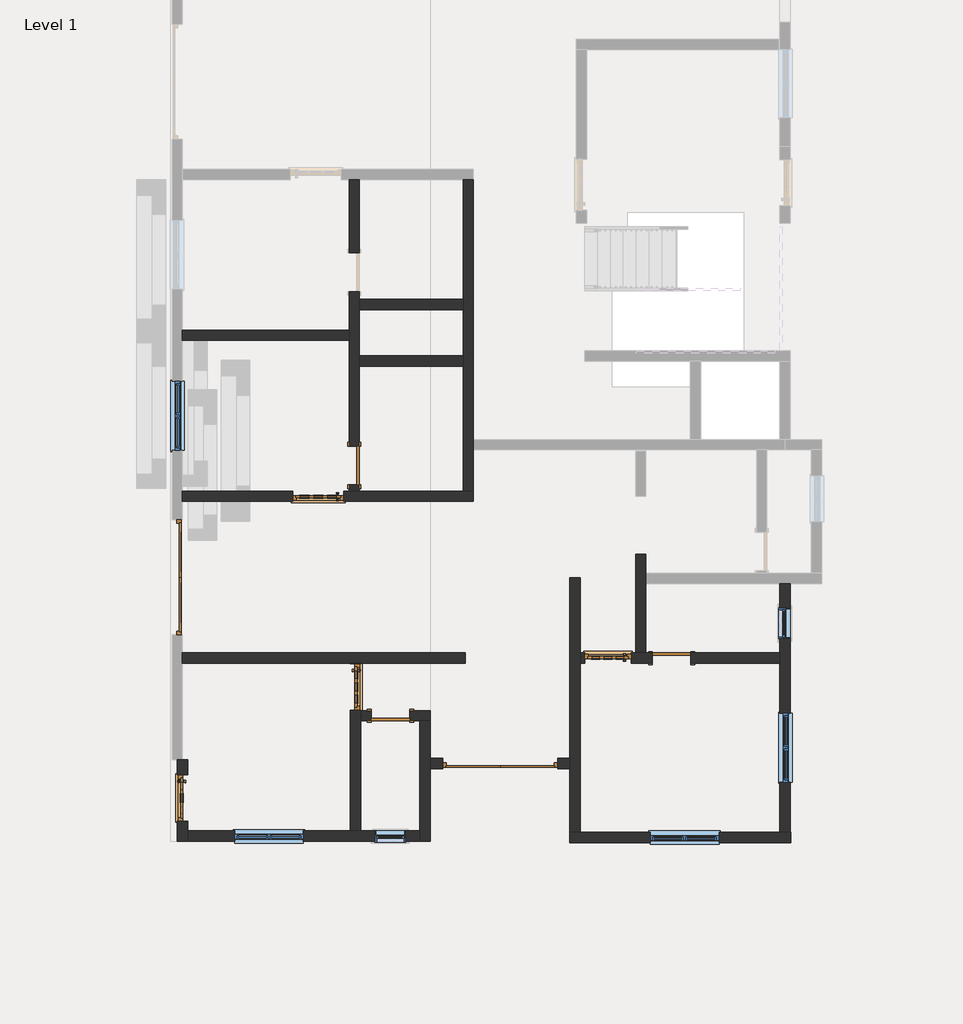
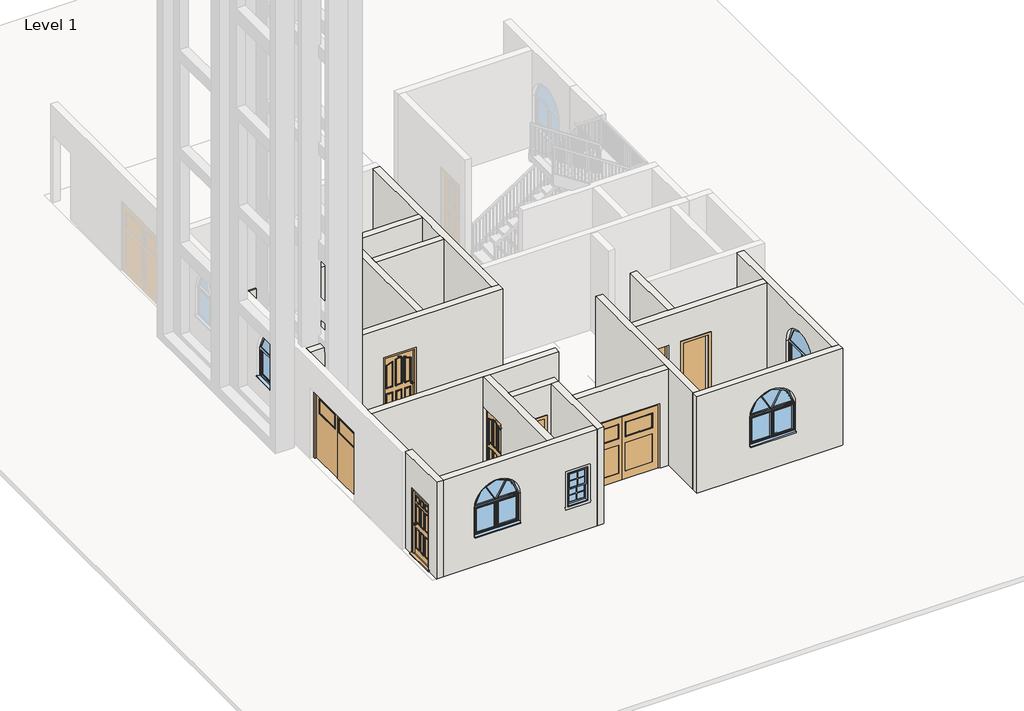
# One storey, part 1 of 4: 18 walls, 9 doors, 6 windows.
"""IFC4 building model written with IfcOpenShell, lengths in millimetres."""

from ifc_helpers import new_model, si_unit, frame, origin, origin_with_axes, place, context, project, spatial, polyline, circle_curve, outline, extrude, faceted_brep, transform, mapped, element, save
from ifc_brep_helpers import plane_surface, revolved_surface, advanced_brep
from components import doors_extsgl_5_910x2110mm_99758a98, doors_extsgl_6_1010x2110mm_b93c615f, doors_extsgl_6_1010x2110mm_efbaf1af, doors_extsgl_6_910x2110mm_72be2df1, doors_extsgl_6_910x2110mm_b26fcae4, doors_extsgl_6_910x2110mm_5dc58899, doors_extsgl_6_910x2110mm_16d7c084, doors_garage_timber_side_hung_glazing_2270x2050mm_ae99176d, doors_garage_timber_side_hung_glazing_2270x2200mm_badb7014, door_fadea3f2, door_53b1b562, window_679d2811, windows_arched_1360x910mm_c5754810

model = new_model("IFC4")

# Units and contexts
model_context = context("Model", 3, world=origin())
ifc_project = project(units=[si_unit("LENGTHUNIT", "METRE", prefix="MILLI")], contexts=[model_context])

# Site, building, storey
site = spatial("IfcSite", under=ifc_project)
building = spatial("IfcBuilding", under=site)
storey = spatial("IfcBuildingStorey", under=building, Name="Level 1", Elevation=0.0)

# Doors
placement = place(None, origin())
doors_extsgl_5_910x2110mm_shape = doors_extsgl_5_910x2110mm_99758a98(model_context)
element("IfcDoor", 1, ObjectType="Doors_ExtSgl_5 : 910x2110mm", at=placement, inside=storey, context=model_context, shape_type="MappedRepresentation", body=[
    mapped(doors_extsgl_5_910x2110mm_shape, transform((-6127.6013636, -9759.5108149, 0.0), x_axis=(0.0, -1.0, 0.0), y_axis=(1.0, 0.0, 0.0), z_axis=(0.0, 0.0, 1.0))),
])
doors_extsgl_6_1010x2110mm_shape = doors_extsgl_6_1010x2110mm_b93c615f(model_context)
doors_extsgl_6_1010x2110mm_2_shape = doors_extsgl_6_1010x2110mm_efbaf1af(model_context)
element("IfcDoor", 2, ObjectType="Doors_ExtSgl_6 : 1010x2110mm", at=placement, inside=storey, context=model_context, shape_type="MappedRepresentation", body=[
    mapped(doors_extsgl_6_1010x2110mm_shape, transform((-3445.8775704, -3805.7037749, 0.0), x_axis=(-1.0, 0.0, 0.0), y_axis=(0.0, -1.0, 0.0), z_axis=(0.0, 0.0, 1.0))),
    mapped(doors_extsgl_6_1010x2110mm_2_shape, transform((-3445.8775704, -3805.7037749, 0.0), x_axis=(-1.0, 0.0, 0.0), y_axis=(0.0, -1.0, 0.0), z_axis=(0.0, 0.0, 1.0))),
])
doors_extsgl_6_910x2110mm_shape = doors_extsgl_6_910x2110mm_72be2df1(model_context)
doors_extsgl_6_910x2110mm_2_shape = doors_extsgl_6_910x2110mm_b26fcae4(model_context)
element("IfcDoor", 3, ObjectType="Doors_ExtSgl_6 : 910x2110mm", at=placement, inside=storey, context=model_context, shape_type="MappedRepresentation", body=[
    mapped(doors_extsgl_6_910x2110mm_shape, transform((2269.1224296, -6998.5466225, 0.0), x_axis=(-1.0, 0.0, 0.0), y_axis=(0.0, -1.0, 0.0), z_axis=(0.0, 0.0, 1.0))),
    mapped(doors_extsgl_6_910x2110mm_2_shape, transform((2269.1224296, -6998.5466225, 0.0), x_axis=(-1.0, 0.0, 0.0), y_axis=(0.0, -1.0, 0.0), z_axis=(0.0, 0.0, 1.0))),
])
doors_extsgl_6_910x2110mm_3_shape = doors_extsgl_6_910x2110mm_5dc58899(model_context)
doors_extsgl_6_910x2110mm_4_shape = doors_extsgl_6_910x2110mm_16d7c084(model_context)
element("IfcDoor", 4, ObjectType="Doors_ExtSgl_6 : 910x2110mm", at=placement, inside=storey, context=model_context, shape_type="MappedRepresentation", body=[
    mapped(doors_extsgl_6_910x2110mm_3_shape, transform((-2709.3109037, -7568.3747197, 0.0), x_axis=(0.0, -1.0, 0.0), y_axis=(1.0, 0.0, 0.0), z_axis=(0.0, 0.0, 1.0))),
    mapped(doors_extsgl_6_910x2110mm_4_shape, transform((-2709.3109037, -7568.3747197, 0.0), x_axis=(0.0, -1.0, 0.0), y_axis=(1.0, 0.0, 0.0), z_axis=(0.0, 0.0, 1.0))),
])
doors_garage_timber_side_hung_glazing_2270x2050mm_shape = doors_garage_timber_side_hung_glazing_2270x2050mm_ae99176d(model_context)
element("IfcDoor", 5, ObjectType="Doors_Garage_Timber_Side_Hung_Glazing : 2270x2050mm", at=placement, inside=storey, context=model_context, shape_type="MappedRepresentation", body=[
    mapped(doors_garage_timber_side_hung_glazing_2270x2050mm_shape, transform((141.8390963, -9078.0694836, 0.0), x_axis=(-1.0, 0.0, 0.0), y_axis=(0.0, -1.0, 0.0), z_axis=(0.0, 0.0, 1.0))),
])
doors_garage_timber_side_hung_glazing_2270x2200mm_shape = doors_garage_timber_side_hung_glazing_2270x2200mm_badb7014(model_context)
element("IfcDoor", 6, ObjectType="Doors_Garage_Timber_Side_Hung_Glazing : 2270x2200mm", at=placement, inside=storey, context=model_context, shape_type="MappedRepresentation", body=[
    mapped(doors_garage_timber_side_hung_glazing_2270x2200mm_shape, transform((-6229.2013636, -5402.1251987, 0.0), x_axis=(0.0, 1.0, 0.0), y_axis=(-1.0, 0.0, 0.0), z_axis=(0.0, 0.0, 1.0))),
])
door_shape = door_fadea3f2(model_context)
element("IfcDoor", 7, ObjectType="Single-Flush : 30\" x 80\"", at=placement, inside=storey, context=model_context, shape_type="MappedRepresentation", body=[
    mapped(door_shape, transform((-2023.5109037, -8138.2694836, 0.0), x_axis=(-1.0, 0.0, 0.0), y_axis=(0.0, -1.0, 0.0), z_axis=(0.0, 0.0, 1.0))),
])
door_2_shape = door_53b1b562(model_context)
element("IfcDoor", 8, ObjectType="Single-Flush : 30\" x 80\"", at=placement, inside=storey, context=model_context, shape_type="MappedRepresentation", body=[
    mapped(door_2_shape, transform((-2734.7109037, -3196.1037749, 0.0), x_axis=(0.0, 1.0, 0.0), y_axis=(-1.0, 0.0, 0.0), z_axis=(0.0, 0.0, 1.0))),
])
element("IfcDoor", 9, ObjectType="Single-Flush : 30\" x 80\"", at=placement, inside=storey, context=model_context, shape_type="MappedRepresentation", body=[
    mapped(door_2_shape, transform((3526.3890963, -6998.5466225, 0.0), x_axis=(-1.0, 0.0, 0.0), y_axis=(0.0, -1.0, 0.0), z_axis=(0.0, 0.0, 1.0))),
])

# Walls
element("IfcWall", 10, ObjectType="Generic - 9\" w", at=placement, inside=storey, context=model_context, shape_type="AdvancedBrep", body=[
    advanced_brep(
    [(1519.7890963, -10638.3037749, 0.0), (5875.8890963, -10638.3037749, 0.0), (5875.8890963, -10638.3037749, 3048.0), (1519.7890963, -10638.3037749, 3048.0), (4460.3890963, -10638.3037749, 914.4), (3100.3890963, -10638.3037749, 914.4), (3100.3890963, -10638.3037749, 1824.4), (4460.3890963, -10638.3037749, 1824.4), (1519.7890963, -10435.1037749, 0.0), (1519.7890963, -10435.1037749, 3048.0), (1722.9890963, -10435.1037749, 3048.0), (5659.9890963, -10435.1037749, 3048.0), (5863.1890963, -10435.1037749, 3048.0), (5875.8890963, -10435.1037749, 3048.0), (5875.8890963, -10435.1037749, 0.0), (5863.1890963, -10435.1037749, 0.0), (5659.9890963, -10435.1037749, 0.0), (1722.9890963, -10435.1037749, 0.0), (4460.3890963, -10435.1037749, 914.4), (4460.3890963, -10435.1037749, 1824.4), (3100.3890963, -10435.1037749, 1824.4), (3100.3890963, -10435.1037749, 914.4)],
    [
        (0, 1),
        (1, 2),
        (2, 3),
        (3, 0),
        (4, 5),
        (5, 6),
        (6, 7, circle_curve(frame((3780.3890963, -10638.3037749, 1824.4), z_axis=(0.0, 1.0, 0.0), x_axis=(-1.0, 0.0, 0.0)), 680.0)),
        (7, 4),
        (8, 9),
        (9, 10),
        (10, 11),
        (11, 12),
        (12, 13),
        (13, 14),
        (14, 15),
        (15, 16),
        (16, 17),
        (17, 8),
        (18, 19),
        (19, 20, circle_curve(frame((3780.3890963, -10435.1037749, 1824.4), z_axis=(0.0, -1.0, 0.0), x_axis=(-1.0, 0.0, 0.0)), 680.0)),
        (20, 21),
        (21, 18),
        (0, 8),
        (14, 1),
        (13, 2),
        (9, 3),
        (18, 4),
        (7, 19),
        (6, 20),
        (5, 21),
    ],
    [
        plane_surface(frame((1722.9890963, -10638.3037749, 0.0), z_axis=(0.0, -1.0, 0.0), x_axis=(1.0, 0.0, 0.0))),
        plane_surface(frame((1722.9890963, -10435.1037749, 0.0), z_axis=(0.0, 1.0, 0.0), x_axis=(-1.0, 0.0, 0.0))),
        plane_surface(frame((1621.3890963, -10638.3037749, 0.0), z_axis=(0.0, 0.0, -1.0), x_axis=(0.0, 1.0, 0.0))),
        plane_surface(frame((5875.8890963, -10638.3037749, 0.0), z_axis=(1.0, 0.0, 0.0), x_axis=(0.0, 1.0, 0.0))),
        plane_surface(frame((5875.8890963, -10638.3037749, 3048.0), z_axis=(0.0, 0.0, 1.0), x_axis=(0.0, 1.0, 0.0))),
        plane_surface(frame((1519.7890963, -5418.6037749, 0.0), z_axis=(-1.0, 0.0, 0.0), x_axis=(0.0, -1.0, 0.0))),
        plane_surface(frame((4460.3890963, -10435.1037749, 914.4), z_axis=(-1.0, 0.0, 0.0), x_axis=(0.0, -1.0, 0.0))),
        revolved_surface(polyline([(3100.3890963, -10638.3037749, 1824.4), (3100.3890963, -10435.1037749, 1824.4)]), (3780.3890963, -10435.1037749, 1824.4), (0.0, -1.0, 0.0)),
        plane_surface(frame((3100.3890963, -10435.1037749, 1824.4), z_axis=(1.0, 0.0, 0.0), x_axis=(0.0, -1.0, 0.0))),
        plane_surface(frame((3100.3890963, -10435.1037749, 914.4), z_axis=(0.0, 0.0, 1.0), x_axis=(0.0, -1.0, 0.0))),
    ],
    [
        (0, [[1, 2, 3, 4], [5, 6, 7, 8]]),
        (1, [[9, 10, 11, 12, 13, 14, 15, 16, 17, 18], [19, 20, 21, 22]]),
        (2, [[-1, 23, -18, -17, -16, -15, 24]]),
        (3, [[-2, -24, -14, 25]]),
        (4, [[-3, -25, -13, -12, -11, -10, 26]]),
        (5, [[-4, -26, -9, -23]]),
        (6, [[-19, 27, -8, 28]]),
        (7, [[-20, -28, -7, 29]]),
        (8, [[-21, -29, -6, 30]]),
        (9, [[-22, -30, -5, -27]]),
    ],
),
])
element("IfcWall", 11, ObjectType="Generic - 9\" w", at=placement, inside=storey, context=model_context, shape_type="AdvancedBrep", body=[
    advanced_brep(
    [(5863.1890963, -10435.1037749, 0.0), (5863.1890963, -5532.9037749, 0.0), (5863.1890963, -5532.9037749, 3048.0), (5863.1890963, -10435.1037749, 3048.0), (5863.1890963, -8087.6251987, 914.4), (5863.1890963, -9447.6251987, 914.4), (5863.1890963, -9447.6251987, 1824.4), (5863.1890963, -8087.6251987, 1824.4), (5863.1890963, -6618.7537749, 1981.2), (5863.1890963, -6009.1537749, 1981.2), (5863.1890963, -6009.1537749, 914.4), (5863.1890963, -6618.7537749, 914.4), (5659.9890963, -10435.1037749, 0.0), (5659.9890963, -10435.1037749, 3048.0), (5659.9890963, -7100.1466225, 3048.0), (5659.9890963, -6896.9466225, 3048.0), (5659.9890963, -5532.9037749, 3048.0), (5659.9890963, -5532.9037749, 0.0), (5659.9890963, -6896.9466225, 0.0), (5659.9890963, -7100.1466225, 0.0), (5659.9890963, -8087.6251987, 914.4), (5659.9890963, -8087.6251987, 1824.4), (5659.9890963, -9447.6251987, 1824.4), (5659.9890963, -9447.6251987, 914.4), (5659.9890963, -6618.7537749, 1981.2), (5659.9890963, -6618.7537749, 914.4), (5659.9890963, -6009.1537749, 914.4), (5659.9890963, -6009.1537749, 1981.2)],
    [
        (0, 1),
        (1, 2),
        (2, 3),
        (3, 0),
        (4, 5),
        (5, 6),
        (6, 7, circle_curve(frame((5863.1890963, -8767.6251987, 1824.4), z_axis=(-1.0, 0.0, 0.0), x_axis=(0.0, -1.0, 0.0)), 680.0)),
        (7, 4),
        (8, 9),
        (9, 10),
        (10, 11),
        (11, 8),
        (12, 13),
        (13, 14),
        (14, 15),
        (15, 16),
        (16, 17),
        (17, 18),
        (18, 19),
        (19, 12),
        (20, 21),
        (21, 22, circle_curve(frame((5659.9890963, -8767.6251987, 1824.4), z_axis=(1.0, 0.0, 0.0), x_axis=(0.0, -1.0, 0.0)), 680.0)),
        (22, 23),
        (23, 20),
        (24, 25),
        (25, 26),
        (26, 27),
        (27, 24),
        (0, 12),
        (17, 1),
        (2, 16),
        (13, 3),
        (20, 4),
        (7, 21),
        (6, 22),
        (5, 23),
        (24, 8),
        (11, 25),
        (10, 26),
        (9, 27),
    ],
    [
        plane_surface(frame((5863.1890963, -10435.1037749, 0.0), z_axis=(1.0, 0.0, 0.0), x_axis=(0.0, 1.0, 0.0))),
        plane_surface(frame((5659.9890963, -10435.1037749, 0.0), z_axis=(-1.0, 0.0, 0.0), x_axis=(0.0, -1.0, 0.0))),
        plane_surface(frame((5863.1890963, -10536.7037749, 0.0), z_axis=(0.0, 0.0, -1.0), x_axis=(-1.0, 0.0, 0.0))),
        plane_surface(frame((5863.1890963, -5431.3037749, 3048.0), z_axis=(0.0, 0.0, 1.0), x_axis=(-1.0, 0.0, 0.0))),
        plane_surface(frame((1722.9890963, -10435.1037749, 0.0), z_axis=(0.0, -1.0, 0.0), x_axis=(-1.0, 0.0, 0.0))),
        plane_surface(frame((3018.3890963, -5532.9037749, 0.0), z_axis=(0.0, 1.0, 0.0), x_axis=(1.0, 0.0, 0.0))),
        plane_surface(frame((5659.9890963, -8087.6251987, 914.4), z_axis=(0.0, -1.0, 0.0), x_axis=(1.0, 0.0, 0.0))),
        revolved_surface(polyline([(5863.1890963, -9447.6251987, 1824.4), (5659.9890963, -9447.6251987, 1824.4)]), (5659.9890963, -8767.6251987, 1824.4), (1.0, 0.0, 0.0)),
        plane_surface(frame((5659.9890963, -9447.6251987, 1824.4), z_axis=(0.0, 1.0, 0.0), x_axis=(1.0, 0.0, 0.0))),
        plane_surface(frame((5659.9890963, -9447.6251987, 914.4), z_axis=(0.0, 0.0, 1.0), x_axis=(1.0, 0.0, 0.0))),
        plane_surface(frame((5659.9890963, -6618.7537749, 1981.2), z_axis=(0.0, 1.0, 0.0), x_axis=(1.0, 0.0, 0.0))),
        plane_surface(frame((5659.9890963, -6618.7537749, 914.4), z_axis=(0.0, 0.0, 1.0), x_axis=(1.0, 0.0, 0.0))),
        plane_surface(frame((5659.9890963, -6009.1537749, 914.4), z_axis=(0.0, -1.0, 0.0), x_axis=(1.0, 0.0, 0.0))),
        plane_surface(frame((5659.9890963, -6009.1537749, 1981.2), z_axis=(0.0, 0.0, -1.0), x_axis=(1.0, 0.0, 0.0))),
    ],
    [
        (0, [[1, 2, 3, 4], [5, 6, 7, 8], [9, 10, 11, 12]]),
        (1, [[13, 14, 15, 16, 17, 18, 19, 20], [21, 22, 23, 24], [25, 26, 27, 28]]),
        (2, [[-1, 29, -20, -19, -18, 30]]),
        (3, [[-3, 31, -16, -15, -14, 32]]),
        (4, [[-4, -32, -13, -29]]),
        (5, [[-2, -30, -17, -31]]),
        (6, [[-21, 33, -8, 34]]),
        (7, [[-22, -34, -7, 35]]),
        (8, [[-23, -35, -6, 36]]),
        (9, [[-24, -36, -5, -33]]),
        (10, [[-25, 37, -12, 38]]),
        (11, [[-26, -38, -11, 39]]),
        (12, [[-27, -39, -10, 40]]),
        (13, [[-28, -40, -9, -37]]),
    ],
),
])
element("IfcWall", 12, ObjectType="Generic - 9\" w", at=placement, inside=storey, context=model_context, shape_type="Brep", body=[
    faceted_brep([(-6229.2013636, -10214.5441482, 2110.0), (-6229.2013636, -10214.5441482, 0.0), (-6229.2013636, -10612.9037749, 0.0), (-6229.2013636, -10612.9037749, 3048.0), (-6229.2013636, -9007.7845215, 3048.0), (-6229.2013636, -9007.7845215, 0.0), (-6229.2013636, -9304.5441482, 0.0), (-6229.2013636, -9304.5441482, 2110.0), (-6026.0013636, -10612.9037749, 0.0), (-6026.0013636, -10409.7037749, 0.0), (-6026.0013636, -10214.5441482, 0.0), (-6026.0013636, -10214.5441482, 2110.0), (-6026.0013636, -9304.5441482, 2110.0), (-6026.0013636, -9304.5441482, 0.0), (-6026.0013636, -9007.7845215, 0.0), (-6026.0013636, -9007.7845215, 3048.0), (-6026.0013636, -10409.7037749, 3048.0), (-6026.0013636, -10612.9037749, 3048.0), (-6127.6013636, -9007.7845215, 0.0), (-6127.6013636, -9007.7845215, 3048.0)], [[[0, 1, 2, 3, 4, 5, 6, 7]], [[8, 9, 10, 11, 12, 13, 14, 15, 16, 17]], [[6, 5, 18, 14, 13]], [[2, 1, 10, 9, 8]], [[4, 3, 17, 16, 15, 19]], [[5, 4, 19, 15, 14, 18]], [[13, 12, 7, 6]], [[11, 10, 1, 0]], [[12, 11, 0, 7]], [[3, 2, 8, 17]]]),
])
element("IfcWall", 13, ObjectType="Generic - 9\" w", at=placement, inside=storey, context=model_context, shape_type="AdvancedBrep", body=[
    advanced_brep(
    [(-6026.0013636, -10612.9037749, 0.0), (-1439.3109037, -10612.9037749, 0.0), (-1439.3109037, -10612.9037749, 3048.0), (-6026.0013636, -10612.9037749, 3048.0), (-3738.4561337, -10612.9037749, 914.4), (-5098.4561337, -10612.9037749, 914.4), (-5098.4561337, -10612.9037749, 1824.4), (-3738.4561337, -10612.9037749, 1824.4), (-1718.7109037, -10612.9037749, 1981.2), (-1718.7109037, -10612.9037749, 914.4), (-2328.3109037, -10612.9037749, 914.4), (-2328.3109037, -10612.9037749, 1981.2), (-6026.0013636, -10409.7037749, 0.0), (-6026.0013636, -10409.7037749, 3048.0), (-2810.9109037, -10409.7037749, 3048.0), (-2607.7109037, -10409.7037749, 3048.0), (-1439.3109037, -10409.7037749, 3048.0), (-1439.3109037, -10409.7037749, 0.0), (-2607.7109037, -10409.7037749, 0.0), (-2810.9109037, -10409.7037749, 0.0), (-3738.4561337, -10409.7037749, 914.4), (-3738.4561337, -10409.7037749, 1824.4), (-5098.4561337, -10409.7037749, 1824.4), (-5098.4561337, -10409.7037749, 914.4), (-1718.7109037, -10409.7037749, 1981.2), (-2328.3109037, -10409.7037749, 1981.2), (-2328.3109037, -10409.7037749, 914.4), (-1718.7109037, -10409.7037749, 914.4)],
    [
        (0, 1),
        (1, 2),
        (2, 3),
        (3, 0),
        (4, 5),
        (5, 6),
        (6, 7, circle_curve(frame((-4418.4561337, -10612.9037749, 1824.4), z_axis=(0.0, 1.0, 0.0), x_axis=(-1.0, 0.0, 0.0)), 680.0)),
        (7, 4),
        (8, 9),
        (9, 10),
        (10, 11),
        (11, 8),
        (12, 13),
        (13, 14),
        (14, 15),
        (15, 16),
        (16, 17),
        (17, 18),
        (18, 19),
        (19, 12),
        (20, 21),
        (21, 22, circle_curve(frame((-4418.4561337, -10409.7037749, 1824.4), z_axis=(0.0, -1.0, 0.0), x_axis=(-1.0, 0.0, 0.0)), 680.0)),
        (22, 23),
        (23, 20),
        (24, 25),
        (25, 26),
        (26, 27),
        (27, 24),
        (0, 12),
        (17, 1),
        (2, 16),
        (13, 3),
        (20, 4),
        (7, 21),
        (6, 22),
        (5, 23),
        (8, 24),
        (27, 9),
        (26, 10),
        (25, 11),
    ],
    [
        plane_surface(frame((-6229.2013636, -10612.9037749, 0.0), z_axis=(0.0, -1.0, 0.0), x_axis=(1.0, 0.0, 0.0))),
        plane_surface(frame((-6229.2013636, -10409.7037749, 0.0), z_axis=(0.0, 1.0, 0.0), x_axis=(-1.0, 0.0, 0.0))),
        plane_surface(frame((-6127.6013636, -10612.9037749, 0.0), z_axis=(0.0, 0.0, -1.0), x_axis=(0.0, 1.0, 0.0))),
        plane_surface(frame((-1337.7109037, -10612.9037749, 3048.0), z_axis=(0.0, 0.0, 1.0), x_axis=(0.0, 1.0, 0.0))),
        plane_surface(frame((-1439.3109037, -8239.8694836, 0.0), z_axis=(1.0, 0.0, 0.0), x_axis=(0.0, -1.0, 0.0))),
        plane_surface(frame((-6026.0013636, -9109.3845215, 0.0), z_axis=(-1.0, 0.0, 0.0), x_axis=(0.0, 1.0, 0.0))),
        plane_surface(frame((-3738.4561337, -10409.7037749, 914.4), z_axis=(-1.0, 0.0, 0.0), x_axis=(0.0, -1.0, 0.0))),
        revolved_surface(polyline([(-5098.4561337, -10612.9037749, 1824.4), (-5098.4561337, -10409.7037749, 1824.4)]), (-4418.4561337, -10409.7037749, 1824.4), (0.0, -1.0, 0.0)),
        plane_surface(frame((-5098.4561337, -10409.7037749, 1824.4), z_axis=(1.0, 0.0, 0.0), x_axis=(0.0, -1.0, 0.0))),
        plane_surface(frame((-5098.4561337, -10409.7037749, 914.4), z_axis=(0.0, 0.0, 1.0), x_axis=(0.0, -1.0, 0.0))),
        plane_surface(frame((-1718.7109037, -10612.9037749, 1981.2), z_axis=(-1.0, 0.0, 0.0), x_axis=(0.0, 1.0, 0.0))),
        plane_surface(frame((-1718.7109037, -10612.9037749, 914.4), z_axis=(0.0, 0.0, 1.0), x_axis=(0.0, 1.0, 0.0))),
        plane_surface(frame((-2328.3109037, -10612.9037749, 914.4), z_axis=(1.0, 0.0, 0.0), x_axis=(0.0, 1.0, 0.0))),
        plane_surface(frame((-2328.3109037, -10612.9037749, 1981.2), z_axis=(0.0, 0.0, -1.0), x_axis=(0.0, 1.0, 0.0))),
    ],
    [
        (0, [[1, 2, 3, 4], [5, 6, 7, 8], [9, 10, 11, 12]]),
        (1, [[13, 14, 15, 16, 17, 18, 19, 20], [21, 22, 23, 24], [25, 26, 27, 28]]),
        (2, [[-1, 29, -20, -19, -18, 30]]),
        (3, [[-3, 31, -16, -15, -14, 32]]),
        (4, [[-2, -30, -17, -31]]),
        (5, [[-4, -32, -13, -29]]),
        (6, [[-21, 33, -8, 34]]),
        (7, [[-22, -34, -7, 35]]),
        (8, [[-23, -35, -6, 36]]),
        (9, [[-24, -36, -5, -33]]),
        (10, [[-9, 37, -28, 38]]),
        (11, [[-10, -38, -27, 39]]),
        (12, [[-11, -39, -26, 40]]),
        (13, [[-12, -40, -25, -37]]),
    ],
),
])
element("IfcWall", 14, ObjectType="Generic -4.5\" p", at=placement, inside=storey, context=model_context, shape_type="Brep", body=[
    faceted_brep([(-2836.3109037, 232.8962251, 0.0), (-2836.3109037, -529.1037749, 0.0), (-2836.3109037, -732.3037749, 0.0), (-2836.3109037, -2815.1037749, 0.0), (-2836.3109037, -2815.1037749, 2032.0), (-2836.3109037, -3577.1037749, 2032.0), (-2836.3109037, -3577.1037749, 0.0), (-2836.3109037, -3704.1037749, 0.0), (-2836.3109037, -3704.1037749, 3048.0), (-2836.3109037, -732.3037749, 3048.0), (-2836.3109037, -529.1037749, 3048.0), (-2836.3109037, 2442.6962251, 3048.0), (-2836.3109037, 2442.6962251, 0.0), (-2836.3109037, 994.8962251, 0.0), (-2836.3109037, 994.8962251, 2032.0), (-2836.3109037, 232.8962251, 2032.0), (-2633.1109037, -2815.1037749, 2032.0), (-2633.1109037, -2815.1037749, 0.0), (-2633.1109037, -1240.3037749, 0.0), (-2633.1109037, -1037.1037749, 0.0), (-2633.1109037, -122.7037749, 0.0), (-2633.1109037, 80.4962251, 0.0), (-2633.1109037, 232.8962251, 0.0), (-2633.1109037, 232.8962251, 2032.0), (-2633.1109037, 994.8962251, 2032.0), (-2633.1109037, 994.8962251, 0.0), (-2633.1109037, 2442.6962251, 0.0), (-2633.1109037, 2442.6962251, 3048.0), (-2633.1109037, 80.4962251, 3048.0), (-2633.1109037, -122.7037749, 3048.0), (-2633.1109037, -1037.1037749, 3048.0), (-2633.1109037, -1240.3037749, 3048.0), (-2633.1109037, -3704.1037749, 3048.0), (-2633.1109037, -3704.1037749, 0.0), (-2633.1109037, -3577.1037749, 0.0), (-2633.1109037, -3577.1037749, 2032.0)], [[[0, 1, 2, 3, 4, 5, 6, 7, 8, 9, 10, 11, 12, 13, 14, 15]], [[16, 17, 18, 19, 20, 21, 22, 23, 24, 25, 26, 27, 28, 29, 30, 31, 32, 33, 34, 35]], [[26, 25, 13, 12]], [[34, 33, 7, 6]], [[22, 21, 20, 19, 18, 17, 3, 2, 1, 0]], [[11, 10, 9, 8, 32, 31, 30, 29, 28, 27]], [[12, 11, 27, 26]], [[8, 7, 33, 32]], [[14, 13, 25, 24]], [[15, 14, 24, 23]], [[0, 15, 23, 22]], [[4, 3, 17, 16]], [[5, 4, 16, 35]], [[6, 5, 35, 34]]]),
])
element("IfcWall", 15, ObjectType="Generic -4.5\" p", at=placement, inside=storey, context=model_context, shape_type="Brep", body=[
    faceted_brep([(-6127.6013636, -3907.3037749, 0.0), (-3950.9109037, -3907.3037749, 0.0), (-3950.9109037, -3907.3037749, 2110.0), (-2940.9109037, -3907.3037749, 2110.0), (-2940.9109037, -3907.3037749, 0.0), (-385.2109037, -3907.3037749, 0.0), (-385.2109037, -3907.3037749, 3048.0), (-6127.6013636, -3907.3037749, 3048.0), (-3950.9109037, -3704.1037749, 2110.0), (-3950.9109037, -3704.1037749, 0.0), (-6127.6013636, -3704.1037749, 0.0), (-6127.6013636, -3704.1037749, 3048.0), (-2836.3109037, -3704.1037749, 3048.0), (-2633.1109037, -3704.1037749, 3048.0), (-588.4109037, -3704.1037749, 3048.0), (-385.2109037, -3704.1037749, 3048.0), (-385.2109037, -3704.1037749, 0.0), (-588.4109037, -3704.1037749, 0.0), (-2633.1109037, -3704.1037749, 0.0), (-2836.3109037, -3704.1037749, 0.0), (-2940.9109037, -3704.1037749, 0.0), (-2940.9109037, -3704.1037749, 2110.0)], [[[0, 1, 2, 3, 4, 5, 6, 7]], [[8, 9, 10, 11, 12, 13, 14, 15, 16, 17, 18, 19, 20, 21]], [[10, 9, 1, 0]], [[20, 19, 18, 17, 16, 5, 4]], [[7, 6, 15, 14, 13, 12, 11]], [[6, 5, 16, 15]], [[4, 3, 21, 20]], [[2, 1, 9, 8]], [[3, 2, 8, 21]], [[0, 7, 11, 10]]]),
])
element("IfcWall", 16, ObjectType="Generic -4.5\" p", at=placement, inside=storey, context=model_context, shape_type="Brep", body=[
    faceted_brep([(-385.2109037, -3704.1037749, 0.0), (-385.2109037, -2891.3037749, 0.0), (-385.2109037, -2688.1037749, 0.0), (-385.2109037, 2442.6962251, 0.0), (-385.2109037, 2442.6962251, 3048.0), (-385.2109037, -2688.1037749, 3048.0), (-385.2109037, -2891.3037749, 3048.0), (-385.2109037, -3704.1037749, 3048.0), (-588.4109037, -3704.1037749, 0.0), (-588.4109037, -3704.1037749, 3048.0), (-588.4109037, -1240.3037749, 3048.0), (-588.4109037, -1037.1037749, 3048.0), (-588.4109037, -122.7037749, 3048.0), (-588.4109037, 80.4962251, 3048.0), (-588.4109037, 2442.6962251, 3048.0), (-588.4109037, 2442.6962251, 0.0), (-588.4109037, 80.4962251, 0.0), (-588.4109037, -122.7037749, 0.0), (-588.4109037, -1037.1037749, 0.0), (-588.4109037, -1240.3037749, 0.0)], [[[0, 1, 2, 3, 4, 5, 6, 7]], [[8, 9, 10, 11, 12, 13, 14, 15, 16, 17, 18, 19]], [[3, 2, 1, 0, 8, 19, 18, 17, 16, 15]], [[7, 6, 5, 4, 14, 13, 12, 11, 10, 9]], [[4, 3, 15, 14]], [[0, 7, 9, 8]]]),
])
element("IfcWall", 17, ObjectType="Generic -4.5\" p", at=placement, inside=storey, context=model_context, shape_type="SweptSolid", body=[
    extrude(outline(polyline([(-588.4109037, -122.7037749), (-2633.1109037, -122.7037749), (-2633.1109037, 80.4962251), (-588.4109037, 80.4962251), (-588.4109037, -122.7037749)])), origin_with_axes(), (0.0, 0.0, 1.0), 3048.0),
])
element("IfcWall", 18, ObjectType="Generic -4.5\" p", at=placement, inside=storey, context=model_context, shape_type="SweptSolid", body=[
    extrude(outline(polyline([(-2836.3109037, -732.3037749), (-6127.6013636, -732.3037749), (-6127.6013636, -529.1037749), (-2836.3109037, -529.1037749), (-2836.3109037, -732.3037749)])), origin_with_axes(), (0.0, 0.0, 1.0), 3048.0),
])
element("IfcWall", 19, ObjectType="Generic -4.5\" p", at=placement, inside=storey, context=model_context, shape_type="SweptSolid", body=[
    extrude(outline(polyline([(-588.4109037, -1240.3037749), (-2633.1109037, -1240.3037749), (-2633.1109037, -1037.1037749), (-588.4109037, -1037.1037749), (-588.4109037, -1240.3037749)])), origin_with_axes(), (0.0, 0.0, 1.0), 3048.0),
])
element("IfcWall", 20, ObjectType="Generic -4.5\" p", at=placement, inside=storey, context=model_context, shape_type="Brep", body=[
    faceted_brep([(-6127.6013636, -7100.1466225, 0.0), (-2810.9109037, -7100.1466225, 0.0), (-2607.7109037, -7100.1466225, 0.0), (-550.3109037, -7100.1466225, 0.0), (-550.3109037, -7100.1466225, 3048.0), (-2607.7109037, -7100.1466225, 3048.0), (-2810.9109037, -7100.1466225, 3048.0), (-6127.6013636, -7100.1466225, 3048.0), (-6127.6013636, -6896.9466225, 0.0), (-6127.6013636, -6896.9466225, 3048.0), (-550.3109037, -6896.9466225, 3048.0), (-550.3109037, -6896.9466225, 0.0)], [[[0, 1, 2, 3, 4, 5, 6, 7]], [[8, 9, 10, 11]], [[3, 2, 1, 0, 8, 11]], [[4, 3, 11, 10]], [[7, 6, 5, 4, 10, 9]], [[0, 7, 9, 8]]]),
])
element("IfcWall", 21, ObjectType="Generic -4.5\" p", at=placement, inside=storey, context=model_context, shape_type="Brep", body=[
    faceted_brep([(-2607.7109037, -10409.7037749, 0.0), (-2607.7109037, -8239.8694836, 0.0), (-2607.7109037, -8036.6694836, 0.0), (-2607.7109037, -8023.4080531, 0.0), (-2607.7109037, -8023.4080531, 2110.0), (-2607.7109037, -7113.4080531, 2110.0), (-2607.7109037, -7113.4080531, 0.0), (-2607.7109037, -7100.1466225, 0.0), (-2607.7109037, -7100.1466225, 3048.0), (-2607.7109037, -8036.6694836, 3048.0), (-2607.7109037, -8239.8694836, 3048.0), (-2607.7109037, -10409.7037749, 3048.0), (-2810.9109037, -8023.4080531, 2110.0), (-2810.9109037, -8023.4080531, 0.0), (-2810.9109037, -10409.7037749, 0.0), (-2810.9109037, -10409.7037749, 3048.0), (-2810.9109037, -7100.1466225, 3048.0), (-2810.9109037, -7100.1466225, 0.0), (-2810.9109037, -7113.4080531, 0.0), (-2810.9109037, -7113.4080531, 2110.0)], [[[0, 1, 2, 3, 4, 5, 6, 7, 8, 9, 10, 11]], [[12, 13, 14, 15, 16, 17, 18, 19]], [[18, 17, 7, 6]], [[14, 13, 3, 2, 1, 0]], [[11, 10, 9, 8, 16, 15]], [[8, 7, 17, 16]], [[6, 5, 19, 18]], [[4, 3, 13, 12]], [[5, 4, 12, 19]], [[0, 11, 15, 14]]]),
])
element("IfcWall", 22, ObjectType="Generic -4.5\" p", at=placement, inside=storey, context=model_context, shape_type="Brep", body=[
    faceted_brep([(-2607.7109037, -8239.8694836, 0.0), (-2404.5109037, -8239.8694836, 0.0), (-2404.5109037, -8239.8694836, 2032.0), (-1642.5109037, -8239.8694836, 2032.0), (-1642.5109037, -8239.8694836, 0.0), (-1439.3109037, -8239.8694836, 0.0), (-1236.1109037, -8239.8694836, 0.0), (-1236.1109037, -8239.8694836, 3048.0), (-1439.3109037, -8239.8694836, 3048.0), (-2607.7109037, -8239.8694836, 3048.0), (-2404.5109037, -8036.6694836, 2032.0), (-2404.5109037, -8036.6694836, 0.0), (-2607.7109037, -8036.6694836, 0.0), (-2607.7109037, -8036.6694836, 3048.0), (-1236.1109037, -8036.6694836, 3048.0), (-1236.1109037, -8036.6694836, 0.0), (-1642.5109037, -8036.6694836, 0.0), (-1642.5109037, -8036.6694836, 2032.0)], [[[0, 1, 2, 3, 4, 5, 6, 7, 8, 9]], [[10, 11, 12, 13, 14, 15, 16, 17]], [[16, 15, 6, 5, 4]], [[12, 11, 1, 0]], [[9, 8, 7, 14, 13]], [[0, 9, 13, 12]], [[7, 6, 15, 14]], [[2, 1, 11, 10]], [[3, 2, 10, 17]], [[4, 3, 17, 16]]]),
])
element("IfcWall", 23, ObjectType="Generic -4.5\" p", at=placement, inside=storey, context=model_context, shape_type="Brep", body=[
    faceted_brep([(-1439.3109037, -8239.8694836, 0.0), (-1439.3109037, -10409.7037749, 0.0), (-1439.3109037, -10612.9037749, 0.0), (-1439.3109037, -10612.9037749, 3048.0), (-1439.3109037, -10409.7037749, 3048.0), (-1439.3109037, -8239.8694836, 3048.0), (-1236.1109037, -8239.8694836, 0.0), (-1236.1109037, -8239.8694836, 3048.0), (-1236.1109037, -8976.4694836, 3048.0), (-1236.1109037, -9179.6694836, 3048.0), (-1236.1109037, -10612.9037749, 3048.0), (-1236.1109037, -10612.9037749, 0.0), (-1236.1109037, -9179.6694836, 0.0), (-1236.1109037, -8976.4694836, 0.0)], [[[0, 1, 2, 3, 4, 5]], [[6, 7, 8, 9, 10, 11, 12, 13]], [[2, 1, 0, 6, 13, 12, 11]], [[5, 4, 3, 10, 9, 8, 7]], [[3, 2, 11, 10]], [[0, 5, 7, 6]]]),
])
element("IfcWall", 24, ObjectType="Generic -4.5\" p", at=placement, inside=storey, context=model_context, shape_type="SweptSolid", body=[
    extrude(outline(polyline([(0.0, -1236.1109037), (0.0, -993.1609037), (2050.0, -993.1609037), (2050.0, 1276.8390963), (0.0, 1276.8390963), (0.0, 1519.7890963), (3048.0, 1519.7890963), (3048.0, -1236.1109037), (0.0, -1236.1109037)])), frame((0.0, -9179.6694836, 0.0), z_axis=(0.0, 1.0, 0.0), x_axis=(0.0, 0.0, 1.0)), (0.0, 0.0, 1.0), 203.2),
])
element("IfcWall", 25, ObjectType="Generic -4.5\" p", at=placement, inside=storey, context=model_context, shape_type="Brep", body=[
    faceted_brep([(1519.7890963, -5418.6037749, 0.0), (1519.7890963, -8976.4694836, 0.0), (1519.7890963, -9179.6694836, 0.0), (1519.7890963, -10435.1037749, 0.0), (1519.7890963, -10435.1037749, 3048.0), (1519.7890963, -9179.6694836, 3048.0), (1519.7890963, -8976.4694836, 3048.0), (1519.7890963, -5418.6037749, 3048.0), (1722.9890963, -5418.6037749, 0.0), (1722.9890963, -5418.6037749, 3048.0), (1722.9890963, -6896.9466225, 3048.0), (1722.9890963, -7100.1466225, 3048.0), (1722.9890963, -10435.1037749, 3048.0), (1722.9890963, -10435.1037749, 0.0), (1722.9890963, -7100.1466225, 0.0), (1722.9890963, -6896.9466225, 0.0)], [[[0, 1, 2, 3, 4, 5, 6, 7]], [[8, 9, 10, 11, 12, 13, 14, 15]], [[3, 2, 1, 0, 8, 15, 14, 13]], [[7, 6, 5, 4, 12, 11, 10, 9]], [[0, 7, 9, 8]], [[4, 3, 13, 12]]]),
])
element("IfcWall", 26, ObjectType="Generic -4.5\" p", at=placement, inside=storey, context=model_context, shape_type="Brep", body=[
    faceted_brep([(2724.0890963, -7100.1466225, 0.0), (3145.3890963, -7100.1466225, 0.0), (3145.3890963, -7100.1466225, 2032.0), (3907.3890963, -7100.1466225, 2032.0), (3907.3890963, -7100.1466225, 0.0), (5659.9890963, -7100.1466225, 0.0), (5659.9890963, -7100.1466225, 3048.0), (1722.9890963, -7100.1466225, 3048.0), (1722.9890963, -7100.1466225, 0.0), (1814.0890963, -7100.1466225, 0.0), (1814.0890963, -7100.1466225, 2110.0), (2724.0890963, -7100.1466225, 2110.0), (3145.3890963, -6896.9466225, 2032.0), (3145.3890963, -6896.9466225, 0.0), (3018.3890963, -6896.9466225, 0.0), (2815.1890963, -6896.9466225, 0.0), (2724.0890963, -6896.9466225, 0.0), (2724.0890963, -6896.9466225, 2110.0), (1814.0890963, -6896.9466225, 2110.0), (1814.0890963, -6896.9466225, 0.0), (1722.9890963, -6896.9466225, 0.0), (1722.9890963, -6896.9466225, 3048.0), (2815.1890963, -6896.9466225, 3048.0), (3018.3890963, -6896.9466225, 3048.0), (5659.9890963, -6896.9466225, 3048.0), (5659.9890963, -6896.9466225, 0.0), (3907.3890963, -6896.9466225, 0.0), (3907.3890963, -6896.9466225, 2032.0)], [[[0, 1, 2, 3, 4, 5, 6, 7, 8, 9, 10, 11]], [[12, 13, 14, 15, 16, 17, 18, 19, 20, 21, 22, 23, 24, 25, 26, 27]], [[20, 19, 9, 8]], [[26, 25, 5, 4]], [[16, 15, 14, 13, 1, 0]], [[7, 6, 24, 23, 22, 21]], [[6, 5, 25, 24]], [[8, 7, 21, 20]], [[0, 11, 17, 16]], [[10, 9, 19, 18]], [[11, 10, 18, 17]], [[2, 1, 13, 12]], [[3, 2, 12, 27]], [[4, 3, 27, 26]]]),
])
element("IfcWall", 27, ObjectType="Generic -4.5\" p", at=placement, inside=storey, context=model_context, shape_type="Brep", body=[
    faceted_brep([(3018.3890963, -6896.9466225, 0.0), (3018.3890963, -5532.9037749, 0.0), (3018.3890963, -5329.7037749, 0.0), (3018.3890963, -4949.7445151, 0.0), (3018.3890963, -4949.7445151, 3048.0), (3018.3890963, -5329.7037749, 3048.0), (3018.3890963, -5532.9037749, 3048.0), (3018.3890963, -6896.9466225, 3048.0), (2815.1890963, -6896.9466225, 0.0), (2815.1890963, -6896.9466225, 3048.0), (2815.1890963, -4949.7445151, 3048.0), (2815.1890963, -4949.7445151, 0.0)], [[[0, 1, 2, 3, 4, 5, 6, 7]], [[8, 9, 10, 11]], [[3, 2, 1, 0, 8, 11]], [[4, 3, 11, 10]], [[7, 6, 5, 4, 10, 9]], [[0, 7, 9, 8]]]),
])

# Windows
window_shape = window_679d2811(model_context)
element("IfcWindow", 28, ObjectType="Window-Double-Hung : 24\" x 42\"", at=placement, inside=storey, context=model_context, shape_type="MappedRepresentation", body=[
    mapped(window_shape, transform((5761.5890963, -6313.9537749, 0.0), x_axis=(0.0, 1.0, 0.0), y_axis=(-1.0, 0.0, 0.0), z_axis=(0.0, 0.0, 1.0))),
])
element("IfcWindow", 29, ObjectType="Window-Double-Hung : 24\" x 42\"", at=placement, inside=storey, context=model_context, shape_type="MappedRepresentation", body=[
    mapped(window_shape, transform((-2023.5109037, -10511.3037749, 0.0), x_axis=(-1.0, 0.0, 0.0), y_axis=(0.0, -1.0, 0.0), z_axis=(0.0, 0.0, 1.0))),
])
windows_arched_1360x910mm_shape = windows_arched_1360x910mm_c5754810(model_context)
element("IfcWindow", 30, ObjectType="Windows_Arched : 1360x910mm", at=placement, inside=storey, context=model_context, shape_type="MappedRepresentation", body=[
    mapped(windows_arched_1360x910mm_shape, transform((-6237.6579314, -2503.2037749, -285.6), x_axis=(0.0, -1.0, 0.0), y_axis=(1.0, 0.0, 0.0), z_axis=(0.0, 0.0, 1.0))),
])
element("IfcWindow", 31, ObjectType="Windows_Arched : 1360x910mm", at=placement, inside=storey, context=model_context, shape_type="MappedRepresentation", body=[
    mapped(windows_arched_1360x910mm_shape, transform((5753.1325284, -9052.6251987, -285.6), x_axis=(0.0, -1.0, 0.0), y_axis=(1.0, 0.0, 0.0), z_axis=(0.0, 0.0, 1.0))),
])
element("IfcWindow", 32, ObjectType="Windows_Arched : 1360x910mm", at=placement, inside=storey, context=model_context, shape_type="MappedRepresentation", body=[
    mapped(windows_arched_1360x910mm_shape, transform((3495.3890963, -10528.2472071, -285.6), x_axis=(-1.0, 0.0, 0.0), y_axis=(0.0, -1.0, 0.0), z_axis=(0.0, 0.0, 1.0))),
])
element("IfcWindow", 33, ObjectType="Windows_Arched : 1360x910mm", at=placement, inside=storey, context=model_context, shape_type="MappedRepresentation", body=[
    mapped(windows_arched_1360x910mm_shape, transform((-4703.4561337, -10502.8472071, -285.6), x_axis=(-1.0, 0.0, 0.0), y_axis=(0.0, -1.0, 0.0), z_axis=(0.0, 0.0, 1.0))),
])

save(model, "model.ifc")

# Revit data of these elements
# Type "Doors_ExtSgl_5 : 910x2110mm"
#   Type Mark = "11"
#   Type Comments = "External Single"
#   Operation = "SingleSwingRight"
#   Construction Type Id = "MDOOR"
#   Keynote = "L20"
#   Analytic Construction = "Metal"
#   Wrap Layers (Int) from Ext = 0' - 6.98819"
#   Wrap Layers (Ext) from Ext = 0' - 4.03543"
#   Thickness = 0' - 1.73228"
#   Stile Top of Lock rail = 3' - 3.37008"
#   Stile Top of Frieze Rail = 5' - 4.96063"
#   Stile Top Rail = 0' - 5.90551"
#   Stile Shutting = 0' - 3.14961"
#   Stile Muntin Rail = 0' - 2.95276"
#   Stile Lock Rail = 0' - 6.88976"
#   Stile Intermediate/Frieze = 0' - 3.14961"
#   Stile Hanging = 0' - 3.14961"
#   Stile Bottom Rail = 0' - 6.88976"
#   Rough Width = 2' - 11.82677"
#   Rough Height = 6' - 11.07087"
#   O/A Frame Width = 0' - 2.51969"
#   Heat Transfer Coefficient (U) = 0.651978 BTU/(h·ft²·°F)
#   Handle Z Distance = 3' - 3.37008"
#   Glazing Thickness = 0' - 0.94488"
#   FrameWidth = 0' - 1.65354"
#   FrameOffset - External = 0' - 0.98425"
#   FrameDepth = 0' - 3.50394"
#   Door Panel Width = 2' - 7.77165"
#   Door Panel Thickness = 0' - 1.73228"
#   Door Panel Height = 6' - 6.74016"
#   DONT CHANGE - Panel Width = 0' - 6.52231"
#   Cill Thickness = 0' - 2.14567"
#   Cill Projection = 0' - 1.1811"
#   Handle X Distance = 0' - 2.95276"
#   Height = 6' - 11.07087"
#   Structural Tolerance = 0' - 0.25591"
#   Tolerance = 0' - 0.11811"
#   Undercut = 0' - 0.15748"
#   Width = 2' - 11.82677"
#   Cill Extension = 0' - 0.98425"
#   Cavity Closer Width = 0' - 1.9685"
#   Cavity Closer Offset from Ext = 0' - 4.03543"
#   Cavity Closer Depth = 0' - 3.34646"
#   Vis - Ironmongery = yes
#   Vis - Cavity Closers = yes
#   Define Thermal Properties by = 1
#   Function = 1
#   Material Glass = Door - Glazing
#   Material Door = Door - Panel
#   Material Frame = Door - Frame/Mullion
#   Material Ironmongery = Door - Handle
#   Visual Light Transmittance = 0
#   Solar Heat Gain Coefficient = 0
#   Wall Closure = (empty or 0)
# Type "Doors_ExtSgl_6 : 1010x2110mm"
#   Type Mark = "12"
#   Type Comments = "External Single"
#   Operation = "SingleSwingRight"
#   Construction Type Id = "SGL"
#   Keynote = "L20"
#   Analytic Construction = "Large single-glazed windows"
#   Wrap Layers (Int) from Ext = 0' - 6.98819"
#   Wrap Layers (Ext) from Ext = 0' - 4.03543"
#   Visual Light Transmittance = 0.9
#   Thickness = 0' - 1.73228"
#   Stile Top of Lock rail = 3' - 3.37008"
#   Stile Top Rail = 0' - 5.90551"
#   Stile Shutting = 0' - 3.54331"
#   Stile Muntin Rail = 0' - 3.54331"
#   Stile Lock Rail = 0' - 6.88976"
#   Stile Hanging = 0' - 3.54331"
#   Stile Bottom Rail = 0' - 6.88976"
#   Solar Heat Gain Coefficient = 0.86
#   Rough Width = 3' - 3.76378"
#   Rough Height = 6' - 11.07087"
#   O/A Frame Width = 0' - 2.51969"
#   Heat Transfer Coefficient (U) = 0.979472 BTU/(h·ft²·°F)
#   Handle Z Distance = 3' - 3.37008"
#   Glazing Thickness = 0' - 0.94488"
#   FrameWidth = 0' - 1.65354"
#   FrameOffset - External = 0' - 0.98425"
#   FrameDepth = 0' - 3.50394"
#   Door Panel Width = 2' - 11.70866"
#   Door Panel Thickness = 0' - 1.73228"
#   Door Panel Height = 6' - 6.74016"
#   DONT CHANGE - Panel Width = 0' - 7.17848"
#   Cill Thickness = 0' - 2.14567"
#   Cill Projection = 0' - 1.1811"
#   Handle X Distance = 0' - 2.95276"
#   Height = 6' - 11.07087"
#   Structural Tolerance = 0' - 0.25591"
#   Tolerance = 0' - 0.11811"
#   Undercut = 0' - 0.15748"
#   Width = 3' - 3.76378"
#   Cill Extension = 0' - 0.98425"
#   Cavity Closer Width = 0' - 1.9685"
#   Cavity Closer Offset from Ext = 0' - 4.03543"
#   Cavity Closer Depth = 0' - 3.34646"
#   Vis - Ironmongery = yes
#   Vis - Cavity Closers = yes
#   Define Thermal Properties by = 1
#   Function = 1
#   Material Glass = Door - Glazing
#   Material Door = Door - Panel
#   Material Frame = Door - Frame/Mullion
#   Material Ironmongery = Door - Handle
#   Wall Closure = (empty or 0)
# Type "Doors_ExtSgl_6 : 910x2110mm"
#   Type Mark = "13"
#   Type Comments = "External Single"
#   Operation = "SingleSwingRight"
#   Construction Type Id = "SGL"
#   Keynote = "L20"
#   Analytic Construction = "Large single-glazed windows"
#   Wrap Layers (Int) from Ext = 0' - 6.98819"
#   Wrap Layers (Ext) from Ext = 0' - 4.03543"
#   Visual Light Transmittance = 0.9
#   Thickness = 0' - 1.73228"
#   Stile Top of Lock rail = 3' - 3.37008"
#   Stile Top Rail = 0' - 5.90551"
#   Stile Shutting = 0' - 3.14961"
#   Stile Muntin Rail = 0' - 2.95276"
#   Stile Lock Rail = 0' - 6.88976"
#   Stile Hanging = 0' - 3.14961"
#   Stile Bottom Rail = 0' - 6.88976"
#   Solar Heat Gain Coefficient = 0.86
#   Rough Width = 2' - 11.82677"
#   Rough Height = 6' - 11.07087"
#   O/A Frame Width = 0' - 2.51969"
#   Heat Transfer Coefficient (U) = 0.979472 BTU/(h·ft²·°F)
#   Handle Z Distance = 3' - 3.37008"
#   Glazing Thickness = 0' - 0.94488"
#   FrameWidth = 0' - 1.65354"
#   FrameOffset - External = 0' - 0.98425"
#   FrameDepth = 0' - 3.50394"
#   Door Panel Width = 2' - 7.77165"
#   Door Panel Thickness = 0' - 1.73228"
#   Door Panel Height = 6' - 6.74016"
#   DONT CHANGE - Panel Width = 0' - 6.52231"
#   Cill Thickness = 0' - 2.14567"
#   Cill Projection = 0' - 1.1811"
#   Handle X Distance = 0' - 2.95276"
#   Height = 6' - 11.07087"
#   Structural Tolerance = 0' - 0.25591"
#   Tolerance = 0' - 0.11811"
#   Undercut = 0' - 0.15748"
#   Width = 2' - 11.82677"
#   Cill Extension = 0' - 0.98425"
#   Cavity Closer Width = 0' - 1.9685"
#   Cavity Closer Offset from Ext = 0' - 4.03543"
#   Cavity Closer Depth = 0' - 3.34646"
#   Vis - Ironmongery = yes
#   Vis - Cavity Closers = yes
#   Define Thermal Properties by = 1
#   Function = 1
#   Material Glass = Door - Glazing
#   Material Door = Door - Panel
#   Material Frame = Door - Frame/Mullion
#   Material Ironmongery = Door - Handle
#   Wall Closure = (empty or 0)
# Type "Doors_Garage_Timber_Side_Hung_Glazing : 2270x2050mm"
#   Type Mark = "8"
#   Type Comments = "External Garage"
#   Operation = "DoubleDoorSingleSwing"
#   Construction Type Id = "GSP4R"
#   Manufacturer = "Revit"
#   Keynote = "L20"
#   Analytic Construction = "1/8 in Pilkington single glazing"
#   Wrap Layers (Ext) from Ext = 0' - 4.03543"
#   Wrap Layers (Int) from Ext = 0' - 6.98819"
#   Visual Light Transmittance = 0.9
#   Thickness = 0' - 1.25984"
#   Stile Top Rail = 0' - 7.87402"
#   Stile Shutting = 0' - 3.93701"
#   Stile Lock Rail = 0' - 7.87402"
#   Stile Hanging = 0' - 6.88976"
#   Stile Bottom Rail = 0' - 9.84252"
#   Solar Heat Gain Coefficient = 0.78
#   Rough Width = 7' - 5.37008"
#   Rough Height = 6' - 8.70866"
#   O/A Frame Width = 0' - 2.51969"
#   Heat Transfer Coefficient (U) = 0.6496 BTU/(h·ft²·°F)
#   Handle Z Distance = 3' - 5.33858"
#   Glazing Panel Height = 1' - 5.71654"
#   FrameWidth = 0' - 1.65354"
#   FrameOffset - External = 0' - 0.98425"
#   FrameDepth = 0' - 3.50394"
#   Door Panel Thickness = 0' - 1.25984"
#   Height = 6' - 8.70866"
#   Structural Tolerance = 0' - 0.31496"
#   Tolerance = 0' - 0.11811"
#   Undercut = 0' - 0.3937"
#   Width = 7' - 5.37008"
#   Cavity Closer Width = 0' - 1.9685"
#   Cavity Closer Offset from Ext = 0' - 4.03543"
#   Cavity Closer Depth = 0' - 3.34646"
#   Vis - Cavity Closers = yes
#   Define Thermal Properties by = 1
#   Function = 1
#   Material Door = Door - Panel
#   Material Frame = Door - Frame/Mullion
#   Material Ironmongery = Door - Handle
#   Wall Closure = (empty or 0)
# Type "Doors_Garage_Timber_Side_Hung_Glazing : 2270x2200mm"
#   Type Mark = "9"
#   Type Comments = "External Garage"
#   Operation = "DoubleDoorSingleSwing"
#   Construction Type Id = "GSP4R"
#   Manufacturer = "Revit"
#   Keynote = "L20"
#   Analytic Construction = "1/8 in Pilkington single glazing"
#   Wrap Layers (Ext) from Ext = 0' - 4.03543"
#   Wrap Layers (Int) from Ext = 0' - 6.98819"
#   Visual Light Transmittance = 0.9
#   Thickness = 0' - 1.25984"
#   Stile Top Rail = 0' - 7.87402"
#   Stile Shutting = 0' - 3.93701"
#   Stile Lock Rail = 0' - 7.87402"
#   Stile Hanging = 0' - 6.88976"
#   Stile Bottom Rail = 0' - 9.84252"
#   Solar Heat Gain Coefficient = 0.78
#   Rough Width = 7' - 5.37008"
#   Rough Height = 7' - 2.61417"
#   O/A Frame Width = 0' - 2.51969"
#   Heat Transfer Coefficient (U) = 0.6496 BTU/(h·ft²·°F)
#   Handle Z Distance = 3' - 5.33858"
#   Glazing Panel Height = 1' - 5.71654"
#   FrameWidth = 0' - 1.65354"
#   FrameOffset - External = 0' - 0.98425"
#   FrameDepth = 0' - 3.50394"
#   Door Panel Thickness = 0' - 1.25984"
#   Height = 7' - 2.61417"
#   Structural Tolerance = 0' - 0.31496"
#   Tolerance = 0' - 0.11811"
#   Undercut = 0' - 0.3937"
#   Width = 7' - 5.37008"
#   Cavity Closer Width = 0' - 1.9685"
#   Cavity Closer Offset from Ext = 0' - 4.03543"
#   Cavity Closer Depth = 0' - 3.34646"
#   Vis - Cavity Closers = yes
#   Define Thermal Properties by = 1
#   Function = 1
#   Material Door = Door - Panel
#   Material Frame = Door - Frame/Mullion
#   Material Ironmongery = Door - Handle
#   Wall Closure = (empty or 0)
# Type "Single-Flush : 30\" x 80\""
#   Type Mark = "5"
#   Construction Type Id = "MDOOR"
#   Assembly Code = "C1020"
#   Analytic Construction = "Metal"
#   Thickness = 0' - 2"
#   Heat Transfer Coefficient (U) = 0.651978 BTU/(h·ft²·°F)
#   Height = 6' - 8"
#   Trim Projection Ext = 0' - 1"
#   Trim Projection Int = 0' - 1"
#   Trim Width = 0' - 3"
#   Width = 2' - 6"
#   Define Thermal Properties by = 1
#   Define Thermal Properties by = 1
#   Door Material = Door - Panel
#   Frame Material = Door - Frame
#   Visual Light Transmittance = 0
#   Solar Heat Gain Coefficient = 0
#   Function = (empty or 0)
#   Wall Closure = (empty or 0)
# Type "Generic - 9\" w"
#   Assembly Code = "B2010"
#   Layers, outside or top first: 0' - 8" no material (function 1)
# Type "Generic -4.5\" p"
#   Assembly Code = "B2010"
#   Layers, outside or top first: 0' - 8" no material (function 1)
# Type "Window-Double-Hung : 24\" x 42\""
#   Type Mark = "10"
#   Fire Rating = "0.5h"
#   Construction Type Id = "DG-DR"
#   Assembly Code = "B2020100"
#   Analytic Construction = "Double glazing - domestic"
#   Wall Thickness [instance default] = 0' - 6"
#   Window Inset [instance default] = 0' - 0"
#   Visual Light Transmittance = 0.81
#   Thermal Resistance (R) = 1.8146 (h·ft²·°F)/BTU
#   Solar Heat Gain Coefficient = 0.76
#   Muntin Width = 1' - 6"
#   Muntin Height = 1' - 5 1/8"
#   Interior Wall Closure [instance default] = 0' - 1 1/2"
#   Rough Width = 2' - 0 1/2"
#   Rough Height = 3' - 6 1/2"
#   Frame Extension [instance default] = 0' - 1 1/4"
#   Exterior Wall Closure [instance default] = 0' - 0 1/2"
#   Extension Jamb [instance default] = 0' - 1 1/2"
#   Heat Transfer Coefficient (U) = 0.5511 BTU/(h·ft²·°F)
#   Height = 3' - 6"
#   Width = 2' - 0"
#   Define Thermal Properties by = 1
#   Top Muntin Visibility = yes
#   Indicator Visibility [instance default] = yes
#   Extension Jamb Visibility [instance default] = yes
#   Interior Trim Visibility [instance default] = yes
#   Exterior Trim Visibility [instance default] = yes
#   Define Thermal Properties by = 1
#   Bottom Muntin Visibility = yes
#   Muntin Pattern = Muntin Pattern_2x2 : Muntin Pattern_2x2
#   Interior Trim Material = Wood - Stained
#   Interior Trim = Trim-Window-Interior-Flat : Picture Frame
#   Exterior Trim Material = Clad - White
#   Exterior Trim = Trim-Window-Exterior-Flat : with Sill
#   Glass Panel Material = Glass
#   Exterior Frame Material = Clad - White
#   Interior Frame Material = Wood - Stained
#   Wall Closure = (empty or 0)
# Type "Windows_Arched : 1360x910mm"
#   Type Mark = "20"
#   Operation = "UserDefined"
#   Construction Type Id = "GSP4R"
#   Manufacturer = "Revit"
#   Keynote = "L10"
#   Analytic Construction = "1/8 in Pilkington single glazing"
#   Wrap Layers (Ext) from Ext = 0' - 4.03543"
#   Wrap Layers (Int) from Ext = 0' - 6.98819"
#   Window Board Projection = 0' - 0.98425"
#   Window Board Extension = 0' - 0.98425"
#   Visual Light Transmittance = 0.9
#   Solar Heat Gain Coefficient = 0.78
#   Rough Width = 4' - 5.54331"
#   Rough Height = 2' - 11.82677"
#   Height = 2' - 11.82677"
#   Width = 4' - 5.54331"
#   Heat Transfer Coefficient (U) = 0.6496 BTU/(h·ft²·°F)
#   Glazing Thickness = 0' - 0.94488"
#   FrameOffset - External = 0' - 1.9685"
#   Frame Depth = 0' - 2.67717"
#   Default Head Height = 6' - 11.07087"
#   Cill Depth = 0' - 3.44488"
#   Cavity Closer Width = 0' - 1.9685"
#   Cavity Closer Offset from Ext = 0' - 4.03543"
#   Cavity Closer Depth = 0' - 3.34646"
#   Vis - Cavity Closers = yes
#   Define Thermal Properties by = 1
#   Material Trim = Window Frame
#   Material Glass = Glass
#   Material Frame = Window Frame
#   Wall Closure = (empty or 0)
# Element 1 (IfcDoor, "Doors_ExtSgl_5 : 910x2110mm")
#   Phase Created = New Construction
#   Materials on its faces: "Door - Panel", "Door - Handle", "Door - Frame/Mullion", "Door - Glazing"
# Element 2 (IfcDoor, "Doors_ExtSgl_6 : 1010x2110mm")
#   Phase Created = New Construction
#   Materials on its faces: "Door - Panel", "Door - Handle", "Door - Frame/Mullion", "Door - Glazing"
# Elements 3, 4 (IfcDoor, "Doors_ExtSgl_6 : 910x2110mm")
#   Phase Created = New Construction
#   Materials on its faces: "Door - Panel", "Door - Handle", "Door - Frame/Mullion", "Door - Glazing"
# Element 5 (IfcDoor, "Doors_Garage_Timber_Side_Hung_Glazing : 2270x2050mm")
#   Phase Created = New Construction
#   Materials on its faces: "Door - Panel", "Door - Frame/Mullion", "Door - Glazing"
# Element 6 (IfcDoor, "Doors_Garage_Timber_Side_Hung_Glazing : 2270x2200mm")
#   Phase Created = New Construction
#   Materials on its faces: "Door - Panel", "Door - Frame/Mullion", "Door - Glazing"
# Elements 7, 8, 9 (IfcDoor, "Single-Flush : 30\" x 80\"")
#   Phase Created = New Construction
#   Materials on its faces: "Door - Frame", "Door - Panel"
# Element 10 (IfcWall, "Generic - 9\" w")
#   Top Offset = 0' - 0"
#   Base Offset = 0' - 0"
#   wall height = 10' - 0"
#   Phase Created = New Construction
#   Base Constraint = Level 1
#   Top Constraint = Level 2
#   Materials on its faces: "Default Wall", "Concrete, Lightweight", "Wood - Stained"
# Element 11 (IfcWall, "Generic - 9\" w")
#   Top Offset = 0' - 0"
#   Base Offset = 0' - 0"
#   wall height = 10' - 0"
#   Phase Created = New Construction
#   Base Constraint = Level 1
#   Top Constraint = Level 2
#   Materials on its faces: "Default Wall", "Wood - Stained"
# Elements 12, 13 (IfcWall, "Generic - 9\" w")
#   Top Offset = 0' - 0"
#   Base Offset = 0' - 0"
#   wall height = 10' - 0"
#   Phase Created = New Construction
#   Base Constraint = Level 1
#   Top Constraint = Level 2
#   Materials on its faces: "Default Wall", "Concrete, Lightweight"
# Elements 14, 15, 16, 17, 18, 19, 20, 21, 22, 25, 26, 27 (IfcWall, "Generic -4.5\" p")
#   Top Offset = 0' - 0"
#   Base Offset = 0' - 0"
#   wall height = 10' - 0"
#   Phase Created = New Construction
#   Base Constraint = Level 1
#   Top Constraint = Level 2
#   Materials on its faces: "Default Wall"
# Element 23 (IfcWall, "Generic -4.5\" p")
#   Top Offset = 0' - 0"
#   Base Offset = 0' - 0"
#   wall height = 10' - 0"
#   Phase Created = New Construction
#   Base Constraint = Level 1
#   Top Constraint = Level 2
#   Materials on its faces: "Default Wall", "Concrete, Lightweight"
# Element 24 (IfcWall, "Generic -4.5\" p")
#   Top Offset = 0' - 0"
#   Base Offset = 0' - 0"
#   wall height = 10' - 0"
#   Phase Created = New Construction
#   Base Constraint = Level 1
#   Top Constraint = Level 2
#   Materials on its faces: "Default Wall", "Door - Frame/Mullion"
# Element 28 (IfcWindow, "Window-Double-Hung : 24\" x 42\"")
#   Mark = "12"
#   Window Inset = 0' - 0"
#   Interior Wall Closure = 0' - 1 1/2"
#   Frame Extension = 0' - 1 1/4"
#   Exterior Wall Closure = 0' - 0 1/2"
#   Interior Trim Visibility = yes
#   Indicator Visibility = yes
#   Exterior Trim Visibility = yes
#   Phase Created = New Construction
#   Materials on its faces: "Wood - Stained", "Glass", "Clad - White"
# Element 29 (IfcWindow, "Window-Double-Hung : 24\" x 42\"")
#   Mark = "82"
#   Window Inset = 0' - 0"
#   Interior Wall Closure = 0' - 1 1/2"
#   Frame Extension = 0' - 1 1/4"
#   Exterior Wall Closure = 0' - 0 1/2"
#   Interior Trim Visibility = yes
#   Indicator Visibility = yes
#   Exterior Trim Visibility = yes
#   Phase Created = New Construction
#   Materials on its faces: "Wood - Stained", "Glass", "Clad - White"
# Element 30 (IfcWindow, "Windows_Arched : 1360x910mm")
#   Mark = "3"
#   Phase Created = New Construction
#   Materials on its faces: "Window Frame", "Glass"
# Element 31 (IfcWindow, "Windows_Arched : 1360x910mm")
#   Mark = "4"
#   Phase Created = New Construction
#   Materials on its faces: "Window Frame", "Glass"
# Element 32 (IfcWindow, "Windows_Arched : 1360x910mm")
#   Mark = "5"
#   Phase Created = New Construction
#   Materials on its faces: "Window Frame", "Glass"
# Element 33 (IfcWindow, "Windows_Arched : 1360x910mm")
#   Mark = "81"
#   Phase Created = New Construction
#   Materials on its faces: "Window Frame", "Glass"
# Materials
#   "Door - Glazing": colour RGB 0 0 255, transparency 0.75
#   "Door - Panel": class "Wood", colour RGB 210 159 95, transparency 0, Cost = 0
#   "Door - Frame/Mullion": class "Wood", colour RGB 212 179 113, transparency 0
#   "Door - Handle": colour RGB 0 0 0, transparency 0
#   "Door - Frame": colour RGB 118 70 51, transparency 0, Cost = 0
#   "Wood - Stained": class "Wood", colour RGB 224 178 126, transparency 0, Cost = 0
#   "Clad - White": class "Wood", colour RGB 242 242 238, transparency 0, Cost = 0
#   "Glass": class "Glass", colour RGB 0 128 192, transparency 0.75, Description = "Soda Lime Glass", Cost = 0
#   "Window Frame": colour RGB 249 249 249, transparency 0
#   "Default Wall": colour RGB 128 128 128, transparency 0, Cost = 0
#   "Concrete, Lightweight": class "Concrete", colour RGB 142 141 140, transparency 0, Description = "Lightweight concrete", Cost = 0
